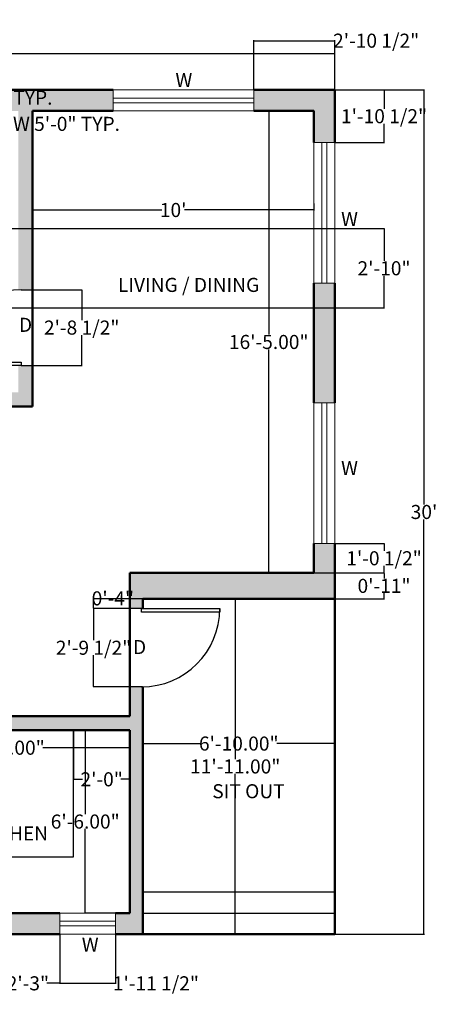
# Model space of a CAD drawing. Units: inches. Extents: x -53 to 395, y -10 to 410.
# Tile 3 of 3: x 217 to 395, y -10 to 410. Entities that reach past the tile are written whole.
import ezdxf

# ---------------------------------------------------------------- set-up
doc = ezdxf.new("R2010")
doc.units = ezdxf.units.IN
doc.header["$MEASUREMENT"] = 0
for name, color, linetype, lineweight in [('A-ANNO-DIMS', 2, 'Continuous', 18), ('A-ANNO-TEXT', 7, 'Continuous', 18), ('A-AREA-IDEN', 7, 'Continuous', 25), ('A-DOOR', 4, 'Continuous', 25), ('A-FLOR-CASE', 8, 'Continuous', 25), ('A-FLOR-STRS', 7, 'Continuous', 25), ('A-GLAZ', 5, 'Continuous', 18), ('A-WALL', 7, 'Continuous', 50)]:
    doc.layers.add(name, color=color, linetype=linetype, lineweight=lineweight)
doc.layers.add('A-WALL-PATT', color=219, linetype='Continuous', lineweight=13, true_color=0x642165)
doc.styles.get("Standard").update_dxf_attribs({"font": 'arial.ttf'})
doc.dimstyles.get("Standard").update_dxf_attribs({"dimtxt": 6, "dimasz": 0.18, "dimexe": 0.18, "dimexo": 0.0625, "dimgap": 0.09, "dimtad": 0, "dimtih": 1, "dimtoh": 1, "dimzin": 0, "dimdsep": 46, "dimlunit": 3, "dimtxsty": 'Standard', "dimcen": 0.09, "dimadec": 0, "dimazin": 0, "dimtfac": 1, "dimtofl": 0, "dimtmove": 0, "dimatfit": 3, "dimfxl": 1, "dimtolj": 1, "dimtzin": 0, "dimarcsym": 0})

# ---------------------------------------------------------------- blocks, each defined once
blk = doc.blocks.new('*U2')
for p, q in [((0, 0), (0, -6)), ((40, 0), (40, -6))]:
    blk.add_line(p, q)
blk.add_lwpolyline([(0, 0), (0, 40), (1.75, 40), (1.75, 0)], close=True)
blk.add_arc((0, 0), 40, 0, 90)
blk = doc.blocks.new('*D8')
at = {"layer": 'A-ANNO-DIMS', "color": 0, "lineweight": -2, "transparency": 16777216}
for p, q in [((27.48, 380.19), (27.48, 395.67)), ((27.66, 395.49), (184.25, 395.49)), ((351.3, 395.49), (194.72, 395.49)), ((351.48, 380.19), (351.48, 395.67))]:
    blk.add_line(p, q, dxfattribs=at)
at = {"layer": 'A-ANNO-DIMS', "color": 0, "transparency": 16777216}
for points in [[(27.66, 395.52), (27.66, 395.46), (27.48, 395.49)], [(351.3, 395.52), (351.3, 395.46), (351.48, 395.49)]]:
    blk.add_solid(points, dxfattribs=at)
at = {"layer": 'Defpoints', "color": 0, "transparency": 16777216}
for p in [(351.48, 395.49), (27.48, 380.13), (351.48, 380.13)]:
    blk.add_point(p, dxfattribs=at)
at = {"layer": 'A-ANNO-DIMS', "color": 0, "transparency": 16777216, "insert": (189.48, 395.49), "char_height": 6, "attachment_point": 5}
blk.add_mtext("\\A1;27'", dxfattribs=at)
blk = doc.blocks.new('*D9')
at = {"layer": 'A-ANNO-DIMS', "color": 0, "lineweight": -2, "transparency": 16777216}
for p, q in [((351.55, 380.13), (389.69, 380.13)), ((389.51, 379.95), (389.51, 203.28)), ((389.51, 20.31), (389.51, 196.97)), ((351.55, 20.13), (389.69, 20.13))]:
    blk.add_line(p, q, dxfattribs=at)
at = {"layer": 'A-ANNO-DIMS', "color": 0, "transparency": 16777216}
for points in [[(389.48, 379.95), (389.54, 379.95), (389.51, 380.13)], [(389.48, 20.31), (389.54, 20.31), (389.51, 20.13)]]:
    blk.add_solid(points, dxfattribs=at)
at = {"layer": 'Defpoints', "color": 0, "transparency": 16777216}
for p in [(351.48, 380.13), (351.48, 20.13), (389.51, 20.13)]:
    blk.add_point(p, dxfattribs=at)
at = {"layer": 'A-ANNO-DIMS', "color": 0, "transparency": 16777216, "insert": (389.51, 200.13), "char_height": 6, "attachment_point": 5}
blk.add_mtext("\\A1;30'", dxfattribs=at)
blk = doc.blocks.new('*D10')
at = {"layer": 'A-ANNO-DIMS', "color": 0, "lineweight": -2, "transparency": 16777216}
for p, q in [((269.48, 105.63), (269.48, 101.21)), ((351.48, 105.63), (351.48, 101.21)), ((269.66, 101.39), (294.24, 101.39)), ((351.3, 101.39), (326.72, 101.39))]:
    blk.add_line(p, q, dxfattribs=at)
at = {"layer": 'A-ANNO-DIMS', "color": 0, "transparency": 16777216}
for points in [[(269.66, 101.42), (269.66, 101.36), (269.48, 101.39)], [(351.3, 101.42), (351.3, 101.36), (351.48, 101.39)]]:
    blk.add_solid(points, dxfattribs=at)
at = {"layer": 'Defpoints', "color": 0, "transparency": 16777216}
for p in [(269.48, 105.69), (351.48, 105.69), (351.48, 101.39)]:
    blk.add_point(p, dxfattribs=at)
at = {"layer": 'A-ANNO-DIMS', "color": 0, "transparency": 16777216, "insert": (310.48, 101.39), "char_height": 6, "attachment_point": 5}
blk.add_mtext('\\A1;6\'-10.00"', dxfattribs=at)
blk = doc.blocks.new('*D11')
at = {"layer": 'A-ANNO-DIMS', "color": 0, "lineweight": -2, "transparency": 16777216}
for p, q in [((351.42, 163.13), (308.79, 163.13)), ((308.97, 162.95), (308.97, 94.78)), ((308.97, 20.31), (308.97, 88.47)), ((351.42, 20.13), (308.79, 20.13))]:
    blk.add_line(p, q, dxfattribs=at)
at = {"layer": 'A-ANNO-DIMS', "color": 0, "transparency": 16777216}
for points in [[(308.94, 162.95), (309, 162.95), (308.97, 163.13)], [(308.94, 20.31), (309, 20.31), (308.97, 20.13)]]:
    blk.add_solid(points, dxfattribs=at)
at = {"layer": 'Defpoints', "color": 0, "transparency": 16777216}
for p in [(308.97, 163.13), (351.48, 163.13), (351.48, 20.13)]:
    blk.add_point(p, dxfattribs=at)
at = {"layer": 'A-ANNO-DIMS', "color": 0, "transparency": 16777216, "insert": (308.97, 91.63), "char_height": 6, "attachment_point": 5}
blk.add_mtext('\\A1;11\'-11.00"', dxfattribs=at)
blk = doc.blocks.new('*D12')
at = {"layer": 'A-ANNO-DIMS', "color": 0, "lineweight": -2, "transparency": 16777216}
for p, q in [((161.98, 107.06), (161.98, 99.44)), ((263.98, 107.06), (263.98, 99.44)), ((162.16, 99.62), (199.09, 99.62)), ((263.8, 99.62), (226.88, 99.62))]:
    blk.add_line(p, q, dxfattribs=at)
at = {"layer": 'A-ANNO-DIMS', "color": 0, "transparency": 16777216}
for points in [[(162.16, 99.65), (162.16, 99.59), (161.98, 99.62)], [(263.8, 99.65), (263.8, 99.59), (263.98, 99.62)]]:
    blk.add_solid(points, dxfattribs=at)
at = {"layer": 'Defpoints', "color": 0, "transparency": 16777216}
for p in [(161.98, 107.13), (263.98, 107.13), (263.98, 99.62)]:
    blk.add_point(p, dxfattribs=at)
at = {"layer": 'A-ANNO-DIMS', "color": 0, "transparency": 16777216, "insert": (212.98, 99.62), "char_height": 6, "attachment_point": 5}
blk.add_mtext('\\A1;8\'-6.00"', dxfattribs=at)
blk = doc.blocks.new('*D20')
at = {"layer": 'A-ANNO-DIMS', "color": 0, "lineweight": -2, "transparency": 16777216}
for p, q in [((342.42, 371.13), (323.08, 371.13)), ((323.26, 370.95), (323.26, 275.78)), ((323.26, 174.31), (323.26, 269.47)), ((342.42, 174.13), (323.08, 174.13))]:
    blk.add_line(p, q, dxfattribs=at)
at = {"layer": 'A-ANNO-DIMS', "color": 0, "transparency": 16777216}
for points in [[(323.23, 370.95), (323.29, 370.95), (323.26, 371.13)], [(323.23, 174.31), (323.29, 174.31), (323.26, 174.13)]]:
    blk.add_solid(points, dxfattribs=at)
at = {"layer": 'Defpoints', "color": 0, "transparency": 16777216}
for p in [(342.48, 371.13), (323.26, 174.13), (342.48, 174.13)]:
    blk.add_point(p, dxfattribs=at)
at = {"layer": 'A-ANNO-DIMS', "color": 0, "transparency": 16777216, "insert": (323.26, 272.63), "char_height": 6, "attachment_point": 5}
blk.add_mtext('\\A1;16\'-5.00"', dxfattribs=at)
blk = doc.blocks.new('*D21')
at = {"layer": 'A-ANNO-DIMS', "color": 0, "lineweight": -2, "transparency": 16777216}
for p, q in [((222.48, 331.64), (222.48, 328.73)), ((222.66, 328.91), (277.58, 328.91)), ((342.3, 328.91), (287.38, 328.91)), ((342.48, 331.64), (342.48, 328.73))]:
    blk.add_line(p, q, dxfattribs=at)
at = {"layer": 'A-ANNO-DIMS', "color": 0, "transparency": 16777216}
for points in [[(222.66, 328.94), (222.66, 328.88), (222.48, 328.91)], [(342.3, 328.94), (342.3, 328.88), (342.48, 328.91)]]:
    blk.add_solid(points, dxfattribs=at)
at = {"layer": 'Defpoints', "color": 0, "transparency": 16777216}
for p in [(222.48, 331.7), (342.48, 331.7), (342.48, 328.91)]:
    blk.add_point(p, dxfattribs=at)
at = {"layer": 'A-ANNO-DIMS', "color": 0, "transparency": 16777216, "insert": (282.48, 328.91), "char_height": 6, "attachment_point": 5}
blk.add_mtext("\\A1;10'", dxfattribs=at)
blk = doc.blocks.new('*D22')
at = {"layer": 'A-ANNO-DIMS', "color": 0, "lineweight": -2, "transparency": 16777216}
for p, q in [((263.92, 107.13), (244.78, 107.13)), ((244.96, 106.95), (244.96, 71.28)), ((244.96, 29.31), (244.96, 64.97)), ((263.92, 29.13), (244.78, 29.13))]:
    blk.add_line(p, q, dxfattribs=at)
at = {"layer": 'A-ANNO-DIMS', "color": 0, "transparency": 16777216}
for points in [[(244.93, 106.95), (244.99, 106.95), (244.96, 107.13)], [(244.93, 29.31), (244.99, 29.31), (244.96, 29.13)]]:
    blk.add_solid(points, dxfattribs=at)
at = {"layer": 'Defpoints', "color": 0, "transparency": 16777216}
for p in [(244.96, 107.13), (263.98, 107.13), (263.98, 29.13)]:
    blk.add_point(p, dxfattribs=at)
at = {"layer": 'A-ANNO-DIMS', "color": 0, "transparency": 16777216, "insert": (244.96, 68.13), "char_height": 6, "attachment_point": 5}
blk.add_mtext('\\A1;6\'-6.00"', dxfattribs=at)
blk = doc.blocks.new('WIN-GLASS-60IN')
for points in [[(60, 2), (0, 2)], [(60, 0), (0, 0)]]:
    blk.add_lwpolyline(points)
blk = doc.blocks.new('*D25')
at = {"layer": 'A-ANNO-DIMS', "color": 0, "lineweight": -2, "transparency": 16777216}
for p, q in [((125.13, 374.56), (125.13, 365.45)), ((185.13, 374.56), (185.13, 365.45)), ((125.31, 365.63), (184.95, 365.63)), ((185.13, 365.63), (185.31, 365.63))]:
    blk.add_line(p, q, dxfattribs=at)
at = {"layer": 'A-ANNO-DIMS', "color": 0, "transparency": 16777216}
for points in [[(125.31, 365.66), (125.31, 365.6), (125.13, 365.63)], [(184.95, 365.66), (184.95, 365.6), (185.13, 365.63)]]:
    blk.add_solid(points, dxfattribs=at)
at = {"layer": 'Defpoints', "color": 0, "transparency": 16777216}
for p in [(125.13, 374.63), (185.13, 374.63), (185.13, 365.63)]:
    blk.add_point(p, dxfattribs=at)
at = {"layer": 'A-ANNO-DIMS', "color": 0, "transparency": 16777216, "insert": (223.36, 365.63), "char_height": 6, "attachment_point": 5}
blk.add_mtext('\\A1;WINDOW 5\'-0" TYP.', dxfattribs=at)
blk = doc.blocks.new('*D26')
at = {"layer": 'A-ANNO-DIMS', "color": 0, "lineweight": -2, "transparency": 16777216}
for p, q in [((185.19, 376.63), (194.31, 376.63)), ((185.19, 374.63), (194.31, 374.63)), ((194.13, 376.63), (194.13, 376.81)), ((194.13, 376.81), (194.31, 376.81)), ((194.13, 374.81), (194.13, 376.45))]:
    blk.add_line(p, q, dxfattribs=at)
at = {"layer": 'A-ANNO-DIMS', "color": 0, "transparency": 16777216}
for points in [[(194.1, 376.45), (194.16, 376.45), (194.13, 376.63)], [(194.1, 374.81), (194.16, 374.81), (194.13, 374.63)]]:
    blk.add_solid(points, dxfattribs=at)
at = {"layer": 'Defpoints', "color": 0, "transparency": 16777216}
for p in [(185.13, 376.63), (185.13, 374.63), (194.13, 376.63)]:
    blk.add_point(p, dxfattribs=at)
at = {"layer": 'A-ANNO-DIMS', "color": 0, "transparency": 16777216, "insert": (212.68, 376.81), "char_height": 6, "attachment_point": 5}
blk.add_mtext('\\A1;0\'-2" TYP.', dxfattribs=at)
blk = doc.blocks.new('*D40')
at = {"layer": 'A-ANNO-DIMS', "color": 0, "lineweight": -2, "transparency": 16777216}
for p, q in [((206.88, 20.06), (206.88, -1.03)), ((234.12, 20.06), (234.12, -1.03)), ((207.06, -0.85), (212.38, -0.85)), ((233.94, -0.85), (228.62, -0.85))]:
    blk.add_line(p, q, dxfattribs=at)
at = {"layer": 'A-ANNO-DIMS', "color": 0, "transparency": 16777216}
for points in [[(207.06, -0.82), (207.06, -0.88), (206.88, -0.85)], [(233.94, -0.82), (233.94, -0.88), (234.12, -0.85)]]:
    blk.add_solid(points, dxfattribs=at)
at = {"layer": 'Defpoints', "color": 0, "transparency": 16777216}
for p in [(206.88, 20.13), (234.12, 20.13), (234.12, -0.85)]:
    blk.add_point(p, dxfattribs=at)
at = {"layer": 'A-ANNO-DIMS', "color": 0, "transparency": 16777216, "insert": (220.5, -0.85), "char_height": 6, "attachment_point": 5}
blk.add_mtext('\\A1;2\'-3"', dxfattribs=at)
blk = doc.blocks.new('*D41')
at = {"layer": 'A-ANNO-DIMS', "color": 0, "lineweight": -2, "transparency": 16777216}
for p, q in [((234.12, 20.06), (234.12, -1.03)), ((257.84, 20.06), (257.84, -1.03)), ((234.3, -0.85), (257.66, -0.85)), ((257.84, -0.85), (258.02, -0.85))]:
    blk.add_line(p, q, dxfattribs=at)
at = {"layer": 'A-ANNO-DIMS', "color": 0, "transparency": 16777216}
for points in [[(234.3, -0.82), (234.3, -0.88), (234.12, -0.85)], [(257.66, -0.82), (257.66, -0.88), (257.84, -0.85)]]:
    blk.add_solid(points, dxfattribs=at)
at = {"layer": 'Defpoints', "color": 0, "transparency": 16777216}
for p in [(234.12, 20.13), (257.84, 20.13), (257.84, -0.85)]:
    blk.add_point(p, dxfattribs=at)
at = {"layer": 'A-ANNO-DIMS', "color": 0, "transparency": 16777216, "insert": (275.12, -0.85), "char_height": 6, "attachment_point": 5}
blk.add_mtext('\\A1;1\'-11 1/2"', dxfattribs=at)
blk = doc.blocks.new('*D43')
at = {"layer": 'A-ANNO-DIMS', "color": 0, "lineweight": -2, "transparency": 16777216}
for p, q in [((316.89, 380.19), (316.89, 401.28)), ((317.07, 401.1), (351.3, 401.1)), ((351.48, 380.19), (351.48, 401.28)), ((351.48, 401.1), (351.66, 401.1))]:
    blk.add_line(p, q, dxfattribs=at)
at = {"layer": 'A-ANNO-DIMS', "color": 0, "transparency": 16777216}
for points in [[(317.07, 401.13), (317.07, 401.07), (316.89, 401.1)], [(351.3, 401.13), (351.3, 401.07), (351.48, 401.1)]]:
    blk.add_solid(points, dxfattribs=at)
at = {"layer": 'Defpoints', "color": 0, "transparency": 16777216}
for p in [(351.48, 401.1), (316.89, 380.13), (351.48, 380.13)]:
    blk.add_point(p, dxfattribs=at)
at = {"layer": 'A-ANNO-DIMS', "color": 0, "transparency": 16777216, "insert": (369.1, 401.1), "char_height": 6, "attachment_point": 5}
blk.add_mtext('\\A1;2\'-10 1/2"', dxfattribs=at)
blk = doc.blocks.new('*D44')
at = {"layer": 'A-ANNO-DIMS', "color": 0, "lineweight": -2, "transparency": 16777216}
for p, q in [((351.55, 380.13), (372.64, 380.13)), ((372.46, 379.95), (372.46, 372.08)), ((372.46, 357.83), (372.46, 365.69)), ((351.55, 357.65), (372.64, 357.65))]:
    blk.add_line(p, q, dxfattribs=at)
at = {"layer": 'A-ANNO-DIMS', "color": 0, "transparency": 16777216}
for points in [[(372.43, 379.95), (372.49, 379.95), (372.46, 380.13)], [(372.43, 357.83), (372.49, 357.83), (372.46, 357.65)]]:
    blk.add_solid(points, dxfattribs=at)
at = {"layer": 'Defpoints', "color": 0, "transparency": 16777216}
for p in [(351.48, 380.13), (372.46, 380.13), (351.48, 357.65)]:
    blk.add_point(p, dxfattribs=at)
at = {"layer": 'A-ANNO-DIMS', "color": 0, "transparency": 16777216, "insert": (372.46, 368.89), "char_height": 6, "attachment_point": 5}
blk.add_mtext('\\A1;1\'-10 1/2"', dxfattribs=at)
blk = doc.blocks.new('*D45')
at = {"layer": 'A-ANNO-DIMS', "color": 0, "lineweight": -2, "transparency": 16777216}
for p, q in [((351.55, 186.68), (372.64, 186.68)), ((372.46, 186.5), (372.46, 183.59)), ((372.46, 174.31), (372.46, 177.21)), ((342.55, 174.13), (372.64, 174.13))]:
    blk.add_line(p, q, dxfattribs=at)
at = {"layer": 'A-ANNO-DIMS', "color": 0, "transparency": 16777216}
for points in [[(372.43, 186.5), (372.49, 186.5), (372.46, 186.68)], [(372.43, 174.31), (372.49, 174.31), (372.46, 174.13)]]:
    blk.add_solid(points, dxfattribs=at)
at = {"layer": 'Defpoints', "color": 0, "transparency": 16777216}
for p in [(351.48, 186.68), (372.46, 186.68), (342.48, 174.13)]:
    blk.add_point(p, dxfattribs=at)
at = {"layer": 'A-ANNO-DIMS', "color": 0, "transparency": 16777216, "insert": (372.46, 180.4), "char_height": 6, "attachment_point": 5}
blk.add_mtext('\\A1;1\'-0 1/2"', dxfattribs=at)
blk = doc.blocks.new('*D46')
at = {"layer": 'A-ANNO-DIMS', "color": 0, "lineweight": -2, "transparency": 16777216}
for p, q in [((27.55, 320.98), (372.64, 320.98)), ((372.46, 320.8), (372.46, 307.21)), ((372.46, 287.31), (372.46, 300.9)), ((36.55, 287.13), (372.64, 287.13))]:
    blk.add_line(p, q, dxfattribs=at)
at = {"layer": 'A-ANNO-DIMS', "color": 0, "transparency": 16777216}
for points in [[(372.43, 320.8), (372.49, 320.8), (372.46, 320.98)], [(372.43, 287.31), (372.49, 287.31), (372.46, 287.13)]]:
    blk.add_solid(points, dxfattribs=at)
at = {"layer": 'Defpoints', "color": 0, "transparency": 16777216}
for p in [(27.48, 320.98), (372.46, 320.98), (36.48, 287.13)]:
    blk.add_point(p, dxfattribs=at)
at = {"layer": 'A-ANNO-DIMS', "color": 0, "transparency": 16777216, "insert": (372.46, 304.05), "char_height": 6, "attachment_point": 5}
blk.add_mtext('\\A1;2\'-10"', dxfattribs=at)
blk = doc.blocks.new('*D50')
at = {"layer": 'A-ANNO-DIMS', "color": 0, "lineweight": -2, "transparency": 16777216}
for p, q in [((222.55, 294.9), (243.64, 294.9)), ((243.46, 294.72), (243.46, 281.95)), ((243.46, 262.81), (243.46, 275.57)), ((222.55, 262.63), (243.64, 262.63))]:
    blk.add_line(p, q, dxfattribs=at)
at = {"layer": 'A-ANNO-DIMS', "color": 0, "transparency": 16777216}
for points in [[(243.43, 294.72), (243.49, 294.72), (243.46, 294.9)], [(243.43, 262.81), (243.49, 262.81), (243.46, 262.63)]]:
    blk.add_solid(points, dxfattribs=at)
at = {"layer": 'Defpoints', "color": 0, "transparency": 16777216}
for p in [(222.48, 294.9), (222.48, 262.63), (243.46, 262.63)]:
    blk.add_point(p, dxfattribs=at)
at = {"layer": 'A-ANNO-DIMS', "color": 0, "transparency": 16777216, "insert": (243.46, 278.76), "char_height": 6, "attachment_point": 5}
blk.add_mtext('\\A1;2\'-8 1/2"', dxfattribs=at)
blk = doc.blocks.new('*D56')
at = {"layer": 'A-ANNO-DIMS', "color": 0, "lineweight": -2, "transparency": 16777216}
for p, q in [((269.42, 158.94), (248.33, 158.94)), ((248.51, 158.76), (248.51, 145.44)), ((248.51, 125.73), (248.51, 139.05)), ((269.42, 125.55), (248.33, 125.55))]:
    blk.add_line(p, q, dxfattribs=at)
at = {"layer": 'A-ANNO-DIMS', "color": 0, "transparency": 16777216}
for points in [[(248.48, 158.76), (248.54, 158.76), (248.51, 158.94)], [(248.48, 125.73), (248.54, 125.73), (248.51, 125.55)]]:
    blk.add_solid(points, dxfattribs=at)
at = {"layer": 'Defpoints', "color": 0, "transparency": 16777216}
for p in [(248.51, 158.94), (269.48, 158.94), (269.48, 125.55)]:
    blk.add_point(p, dxfattribs=at)
at = {"layer": 'A-ANNO-DIMS', "color": 0, "transparency": 16777216, "insert": (248.51, 142.24), "char_height": 6, "attachment_point": 5}
blk.add_mtext('\\A1;2\'-9 1/2"', dxfattribs=at)
blk = doc.blocks.new('*D57')
at = {"layer": 'A-ANNO-DIMS', "color": 0, "lineweight": -2, "transparency": 16777216}
for p, q in [((269.42, 163.13), (248.33, 163.13)), ((248.51, 163.13), (248.51, 163.31)), ((248.51, 163.31), (248.69, 163.31)), ((248.51, 159.12), (248.51, 162.95)), ((269.42, 158.94), (248.33, 158.94))]:
    blk.add_line(p, q, dxfattribs=at)
at = {"layer": 'A-ANNO-DIMS', "color": 0, "transparency": 16777216}
for points in [[(248.48, 162.95), (248.54, 162.95), (248.51, 163.13)], [(248.48, 159.12), (248.54, 159.12), (248.51, 158.94)]]:
    blk.add_solid(points, dxfattribs=at)
at = {"layer": 'Defpoints', "color": 0, "transparency": 16777216}
for p in [(248.51, 163.13), (269.48, 163.13), (269.48, 158.94)]:
    blk.add_point(p, dxfattribs=at)
at = {"layer": 'A-ANNO-DIMS', "color": 0, "transparency": 16777216, "insert": (256.75, 163.31), "char_height": 6, "attachment_point": 5}
blk.add_mtext('\\A1;0\'-4"', dxfattribs=at)
blk = doc.blocks.new('*D58')
at = {"layer": 'A-ANNO-DIMS', "color": 0, "lineweight": -2, "transparency": 16777216}
for p, q in [((342.55, 174.13), (372.64, 174.13)), ((372.46, 173.95), (372.46, 171.78)), ((372.46, 163.31), (372.46, 165.47)), ((351.55, 163.13), (372.64, 163.13))]:
    blk.add_line(p, q, dxfattribs=at)
at = {"layer": 'A-ANNO-DIMS', "color": 0, "transparency": 16777216}
for points in [[(372.43, 173.95), (372.49, 173.95), (372.46, 174.13)], [(372.43, 163.31), (372.49, 163.31), (372.46, 163.13)]]:
    blk.add_solid(points, dxfattribs=at)
at = {"layer": 'Defpoints', "color": 0, "transparency": 16777216}
for p in [(342.48, 174.13), (351.48, 163.13), (372.46, 163.13)]:
    blk.add_point(p, dxfattribs=at)
at = {"layer": 'A-ANNO-DIMS', "color": 0, "transparency": 16777216, "insert": (372.46, 168.63), "char_height": 6, "attachment_point": 5}
blk.add_mtext('\\A1;0\'-11"', dxfattribs=at)
blk = doc.blocks.new('*D63')
at = {"layer": 'A-ANNO-DIMS', "color": 0, "lineweight": -2, "transparency": 16777216}
for p, q in [((239.98, 107.06), (239.98, 85.97)), ((263.98, 107.06), (263.98, 85.97)), ((240.16, 86.15), (243.87, 86.15)), ((263.8, 86.15), (260.1, 86.15))]:
    blk.add_line(p, q, dxfattribs=at)
at = {"layer": 'A-ANNO-DIMS', "color": 0, "transparency": 16777216}
for points in [[(240.16, 86.18), (240.16, 86.12), (239.98, 86.15)], [(263.8, 86.18), (263.8, 86.12), (263.98, 86.15)]]:
    blk.add_solid(points, dxfattribs=at)
at = {"layer": 'Defpoints', "color": 0, "transparency": 16777216}
for p in [(239.98, 107.13), (263.98, 107.13), (239.98, 86.15)]:
    blk.add_point(p, dxfattribs=at)
at = {"layer": 'A-ANNO-DIMS', "color": 0, "transparency": 16777216, "insert": (251.98, 86.15), "char_height": 6, "attachment_point": 5}
blk.add_mtext('\\A1;2\'-0"', dxfattribs=at)

msp = doc.modelspace()

# ---------------------------------------------------------------- hatches: boundary and pattern name
at = {"layer": 'A-WALL-PATT'}
h = msp.add_hatch(color=256, dxfattribs=at)
h.dxf.hatch_style = 1
h.paths.add_polyline_path([(36.483, 371.127), (84.483, 371.127), (84.483, 365.369), (86.914, 365.369), (90.483, 365.369), (90.483, 371.127), (125.127, 371.127), (125.127, 380.127), (27.483, 380.127), (27.483, 344.976), (36.483, 344.976)])
h.paths.add_polyline_path([(256.886, 380.127), (185.127, 380.127), (185.127, 371.127), (216.483, 371.127), (216.483, 294.874, -0.0089901), (217.643, 294.895), (222.483, 294.895), (222.483, 371.127), (256.886, 371.127)])
h.paths.add_polyline_path([(351.483, 380.127), (316.886, 380.127), (316.886, 371.127), (342.483, 371.127), (342.483, 370.595), (342.483, 357.645), (351.483, 357.645)])
h.paths.add_polyline_path([(351.483, 297.645), (342.483, 297.645), (342.483, 246.678), (351.483, 246.678)])
h.paths.add_polyline_path([(351.483, 186.678), (342.483, 186.678), (342.483, 174.127), (263.983, 174.127), (263.983, 158.936), (268.991, 158.936), (269.483, 158.936), (269.483, 163.127), (351.483, 163.127)])
h.paths.add_polyline_path([(90.483, 245.127), (84.483, 245.127), (84.483, 173.127), (90.483, 173.127)])
h = msp.add_hatch(color=256, dxfattribs=at)
h.dxf.hatch_style = 1
h.paths.add_polyline_path([(90.483, 278.924), (90.482, 278.924), (90.482, 338.924), (90.482, 341.579), (86.914, 341.579, -0.0256023), (84.483, 341.703), (84.483, 287.127), (36.467, 287.127), (36.467, 320.976), (27.483, 320.976), (27.483, 224.19), (36.483, 224.19), (36.483, 281.127), (84.483, 281.127), (84.483, 251.127), (36.483, 251.127), (36.483, 245.127), (222.483, 245.127), (222.483, 262.629), (217.643, 262.629), (216.483, 262.629), (216.483, 251.127), (90.483, 251.127)])
h = msp.add_hatch(color=256, dxfattribs=at)
h.dxf.hatch_style = 1
h.paths.add_polyline_path([(36.482, 120.321), (36.483, 167.127), (61.404, 167.127), (61.404, 170.14, -0.0373537), (61.627, 173.127), (36.483, 173.127), (36.483, 200.19), (27.483, 200.19), (27.483, 20.127), (70.241, 20.127), (70.241, 29.127), (36.483, 29.127), (36.483, 60.321), (36.482, 60.321)])
h.paths.add_polyline_path([(161.983, 173.127), (81.484, 173.127), (81.484, 170.14), (81.484, 167.127), (156.483, 167.127), (156.483, 160.02), (156.768, 160.02), (161.983, 160.02)])
h.paths.add_polyline_path([(161.983, 107.127), (263.983, 107.127), (263.983, 29.127), (257.837, 29.127), (257.837, 20.127), (264.483, 20.127), (269.483, 20.127), (269.483, 125.551, -0.003682), (268.991, 125.548), (263.983, 125.548), (263.983, 113.127), (161.983, 113.127), (161.983, 125.256), (156.483, 125.256), (156.483, 29.127), (118.241, 29.127), (118.241, 20.127), (170.876, 20.127), (170.876, 29.127), (161.983, 29.127)])
h.paths.add_polyline_path([(140.509, 61.902), (171.852, 61.902), (171.852, 74.267), (140.509, 74.267)], flags=25)
h = msp.add_hatch(color=256, dxfattribs=at)
h.dxf.hatch_style = 1
h.paths.add_polyline_path([(161.983, 107.127), (263.983, 107.127), (263.983, 29.127), (257.837, 29.127), (257.837, 20.127), (264.483, 20.127), (269.483, 20.127), (269.483, 125.551, -0.003682), (268.991, 125.548), (263.983, 125.548), (263.983, 113.127), (161.983, 113.127), (161.983, 125.256), (156.768, 125.256, -0.0020525), (156.483, 125.257), (156.483, 29.127), (118.241, 29.127), (118.241, 20.127), (170.876, 20.127), (170.876, 29.127), (161.983, 29.127)])
h = msp.add_hatch(color=256, dxfattribs=at)
h.dxf.hatch_style = 1
h.paths.add_polyline_path([(234.123, 29.127), (206.876, 29.127), (206.876, 20.127), (234.123, 20.127)])

# ---------------------------------------------------------------- linework, layer by layer
at = {"layer": 'A-FLOR-CASE'}
for points in [[(239.983, 53.127), (239.983, 107.127)], [(161.983, 53.127), (239.983, 53.127)]]:
    msp.add_lwpolyline(points, dxfattribs=at)
at = {"layer": 'A-FLOR-STRS'}
for points in [[(269.483, 38.127), (351.483, 38.127)], [(269.483, 29.127), (351.483, 29.127)]]:
    msp.add_lwpolyline(points, dxfattribs=at)
at = {"layer": 'A-GLAZ'}
for points in [[(256.886, 380.127), (316.886, 380.127), (316.886, 371.127), (256.886, 371.127)], [(342.483, 357.645), (351.483, 357.645), (351.483, 297.645), (342.483, 297.645)], [(342.483, 246.678), (351.483, 246.678), (351.483, 186.678), (342.483, 186.678)], [(234.123, 29.127), (257.837, 29.127), (257.837, 20.127), (234.123, 20.127)]]:
    msp.add_lwpolyline(points, close=True, dxfattribs=at)
for points in [[(234.123, 25.627), (257.837, 25.627)], [(234.123, 23.627), (257.837, 23.627)]]:
    msp.add_lwpolyline(points, dxfattribs=at)
at = {"layer": 'A-WALL'}
for points in [[(256.886, 380.127), (185.127, 380.127)], [(351.483, 380.127), (316.886, 380.127)], [(351.483, 357.645), (351.483, 380.127)], [(222.483, 245.127), (222.483, 371.127)], [(256.886, 371.127), (222.483, 371.127)], [(256.886, 371.127), (222.483, 371.127)], [(342.483, 370.595), (342.483, 371.127), (316.886, 371.127)], [(342.483, 357.645), (342.483, 370.595)], [(342.483, 246.678), (342.483, 297.645)], [(351.483, 246.678), (351.483, 297.645)], [(222.483, 245.127), (36.483, 245.127)], [(342.483, 174.127), (342.483, 186.678)], [(342.483, 174.127), (342.483, 186.678)], [(351.483, 20.127), (351.483, 186.678)], [(342.483, 174.127), (263.983, 174.127)], [(263.983, 113.127), (263.983, 174.127)], [(269.483, 163.127), (351.483, 163.127)], [(269.483, 158.936), (269.483, 163.127)], [(269.483, 20.127), (269.483, 125.551)], [(161.983, 113.127), (263.983, 113.127)], [(161.983, 107.127), (263.983, 107.127)], [(263.983, 29.127), (263.983, 107.127)], [(206.876, 29.127), (234.123, 29.127)], [(257.837, 29.127), (263.983, 29.127)], [(206.876, 20.127), (234.123, 20.127)], [(257.837, 20.127), (264.483, 20.127)], [(264.483, 20.127), (351.483, 20.127)]]:
    msp.add_lwpolyline(points, dxfattribs=at)

# ---------------------------------------------------------------- block references
at = {"layer": 'A-DOOR'}
for p, xscale, yscale, zscale, rotation in [((217.643, 262.629), 0.8066612292799318, 0.8066612292799318, 0.8066612292799318, 90), ((268.991, 158.936), 0.8347114754771883, 0.8347114754771883, 0.8347114754771883, 270)]:
    msp.add_blockref('*U2', p, dxfattribs=dict(at, xscale=xscale, yscale=yscale, zscale=zscale, rotation=rotation))
at = {"layer": 'A-GLAZ'}
msp.add_blockref('WIN-GLASS-60IN', (256.886, 374.627), dxfattribs=at)
for p, rotation in [((345.982, 357.646), 270), ((347.983, 186.677), 90.00000000000003)]:
    msp.add_blockref('WIN-GLASS-60IN', p, dxfattribs=dict(at, rotation=rotation))

# ---------------------------------------------------------------- texts
at = {"layer": 'A-ANNO-TEXT', "char_height": 6, "attachment_point": 1}
for s, insert in [('W', (283.461, 387.31)), ('W', (354.136, 328.049)), ('D', (216.682, 282.943)), ('W', (354.136, 221.839)), ('D', (265.337, 145.528)), ('W', (243.491, 18.667))]:
    msp.add_mtext_dynamic_manual_height_columns(s, width=74.47502, gutter_width=1, heights=[0], dxfattribs=dict(at, insert=insert))
at = {"layer": 'A-AREA-IDEN', "char_height": 6, "attachment_point": 1}
for s, insert in [('LIVING / DINING', (258.932, 299.962)), ('SIT OUT', (299.18, 84.07)), ('KITCHEN ', (194.607, 66.055))]:
    msp.add_mtext_dynamic_manual_height_columns(s, width=74.47502, gutter_width=1, heights=[0], dxfattribs=dict(at, insert=insert))

# ---------------------------------------------------------------- dimensions: what is measured, and where the dimension line sits
at = {"layer": 'A-ANNO-DIMS'}
for base, p1, p2, override, picture, middle in [((351.483, 401.102), (316.886, 380.127), (351.483, 380.127), {"dimdec": 1, "dimlfac": 1, "dimrnd": 0, "dimzin": 1, "dimdsep": 46, "dimlunit": 4, "dimfrac": 2}, '*D43', (369.1, 401.102)), ((351.483, 395.485), (27.483, 380.127), (351.483, 380.127), {"dimclrd": 0, "dimclre": 0, "dimclrt": 0}, '*D8', (189.483, 395.485)), ((342.483, 328.915), (222.483, 331.7), (342.483, 331.7), {"dimclrd": 0, "dimclre": 0, "dimclrt": 0}, '*D21', (282.483, 328.915)), ((263.983, 99.62), (161.983, 107.127), (263.983, 107.127), {"dimclrd": 0, "dimclre": 0, "dimclrt": 0}, '*D12', (212.983, 99.62)), ((351.483, 101.386), (269.483, 105.688), (351.483, 105.688), {"dimclrd": 0, "dimclre": 0, "dimclrt": 0}, '*D10', (310.483, 101.386)), ((234.123, -0.848), (206.876, 20.127), (234.123, 20.127), {"dimdec": 1, "dimlfac": 1, "dimrnd": 0, "dimzin": 1, "dimdsep": 46, "dimlunit": 4, "dimfrac": 2}, '*D40', (220.5, -0.848)), ((257.837, -0.848), (234.123, 20.127), (257.837, 20.127), {"dimdec": 1, "dimlfac": 1, "dimrnd": 0, "dimzin": 1, "dimdsep": 46, "dimlunit": 4, "dimfrac": 2}, '*D41', (275.121, -0.848))]:
    dim = msp.add_linear_dim(base=base, p1=p1, p2=p2, dimstyle='Standard', override=override, dxfattribs=at)
    dim.commit()
    dim.dimension.update_dxf_attribs({"geometry": picture, "text_midpoint": middle})
dim = msp.add_linear_dim(base=(194.127, 376.627), p1=(185.127, 374.627), p2=(185.127, 376.627), angle=90, text='<> TYP.', dimstyle='Standard', override={"dimdec": 1, "dimlfac": 1, "dimrnd": 0, "dimzin": 1, "dimdsep": 46, "dimlunit": 4, "dimfrac": 2}, dxfattribs=at)
dim.commit()
dim.dimension.update_dxf_attribs({"geometry": '*D26', "text_midpoint": (212.684, 376.807)})
dim = msp.add_linear_dim(base=(185.127, 365.627), p1=(125.127, 374.627), p2=(185.127, 374.627), text='WINDOW <> TYP.', dimstyle='Standard', override={"dimdec": 1, "dimlfac": 1, "dimrnd": 0, "dimzin": 1, "dimdsep": 46, "dimlunit": 4, "dimfrac": 2}, dxfattribs=at)
dim.commit()
dim.dimension.update_dxf_attribs({"geometry": '*D25', "text_midpoint": (223.36, 365.627)})
for base, p1, p2, angle, override, picture, middle in [((389.513, 20.127), (351.483, 380.127), (351.483, 20.127), 90, {"dimclrd": 0, "dimclre": 0, "dimclrt": 0}, '*D9', (389.513, 200.127)), ((372.458, 380.127), (351.483, 357.645), (351.483, 380.127), 90, {"dimdec": 1, "dimlfac": 1, "dimrnd": 0, "dimzin": 1, "dimdsep": 46, "dimlunit": 4, "dimfrac": 2}, '*D44', (372.458, 368.886)), ((323.258, 174.127), (342.483, 371.127), (342.483, 174.127), 90, {"dimclrd": 0, "dimclre": 0, "dimclrt": 0}, '*D20', (323.258, 272.627)), ((372.458, 320.976), (36.483, 287.127), (27.483, 320.976), 90, {"dimdec": 1, "dimlfac": 1, "dimrnd": 0, "dimzin": 1, "dimdsep": 46, "dimlunit": 4, "dimfrac": 2}, '*D46', (372.458, 304.052)), ((243.458, 262.629), (222.483, 294.895), (222.483, 262.629), 270, {"dimdec": 1, "dimlfac": 1, "dimrnd": 0, "dimzin": 1, "dimdsep": 46, "dimlunit": 4, "dimfrac": 2}, '*D50', (243.458, 278.762)), ((372.458, 186.678), (342.483, 174.127), (351.483, 186.678), 90, {"dimdec": 1, "dimlfac": 1, "dimrnd": 0, "dimzin": 1, "dimdsep": 46, "dimlunit": 4, "dimfrac": 2}, '*D45', (372.458, 180.403)), ((372.458, 163.127), (342.483, 174.127), (351.483, 163.127), 90, {"dimdec": 1, "dimlfac": 1, "dimrnd": 0, "dimzin": 1, "dimdsep": 46, "dimlunit": 4, "dimfrac": 2}, '*D58', (372.458, 168.627)), ((248.508, 163.127), (269.483, 158.936), (269.483, 163.127), 90, {"dimdec": 1, "dimlfac": 1, "dimrnd": 0, "dimzin": 1, "dimdsep": 46, "dimlunit": 4, "dimfrac": 2}, '*D57', (256.752, 163.307)), ((308.974, 163.127), (351.483, 20.127), (351.483, 163.127), 90, {"dimclrd": 0, "dimclre": 0, "dimclrt": 0}, '*D11', (308.974, 91.627)), ((248.508, 158.936), (269.483, 125.551), (269.483, 158.936), 90, {"dimdec": 1, "dimlfac": 1, "dimrnd": 0, "dimzin": 1, "dimdsep": 46, "dimlunit": 4, "dimfrac": 2}, '*D56', (248.508, 142.244)), ((244.956, 107.127), (263.983, 29.127), (263.983, 107.127), 90, {"dimclrd": 0, "dimclre": 0, "dimclrt": 0}, '*D22', (244.956, 68.127)), ((239.983, 86.152), (263.983, 107.127), (239.983, 107.127), 180, {"dimdec": 1, "dimlfac": 1, "dimrnd": 0, "dimzin": 1, "dimdsep": 46, "dimlunit": 4, "dimfrac": 2}, '*D63', (251.983, 86.152))]:
    dim = msp.add_linear_dim(base=base, p1=p1, p2=p2, angle=angle, dimstyle='Standard', override=override, dxfattribs=at)
    dim.commit()
    dim.dimension.update_dxf_attribs({"geometry": picture, "text_midpoint": middle})

doc.saveas('drawing.dxf')
